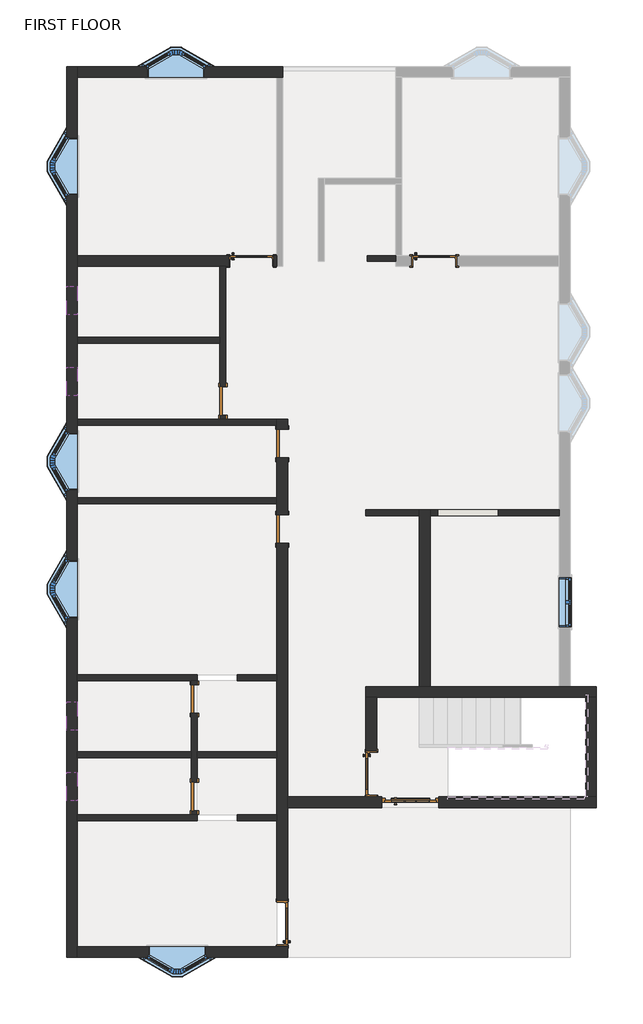
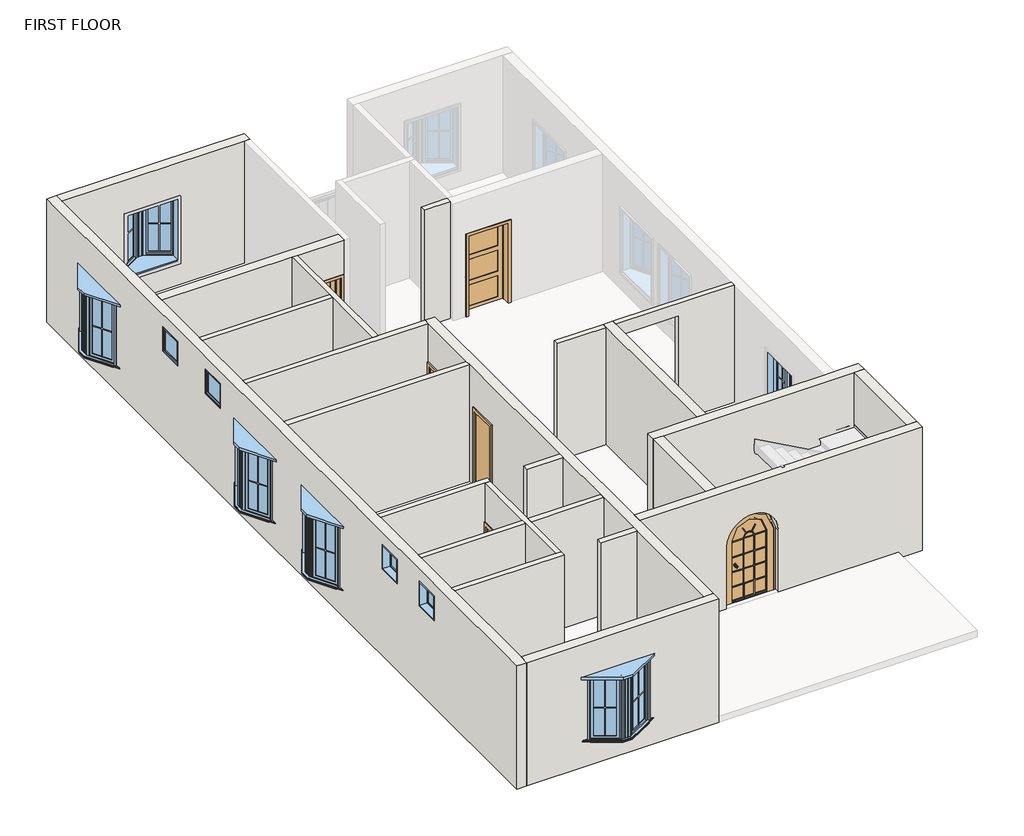
# One storey, part 1 of 2: 23 walls, 10 doors, 10 windows.
"""IFC4 building model written with IfcOpenShell, lengths in millimetres."""

from ifc_helpers import new_model, si_unit, frame, origin, place, context, project, spatial, polyline, circle_curve, outline, extrude, faceted_brep, transform, mapped, element, save
from ifc_brep_helpers import plane_surface, revolved_surface, advanced_brep
from components import door_interior_single_3_panel_vert_wood_interior_door_3_x_7_9905b5e2, door_interior_single_3_panel_vert_wood_interior_door_3_x_7_d98c575a, door_arched_single_french_glass_wood_exterior_1219_x_2134mm_7a906126, single_flush_bathroom_flush_door_2_x_7_025d1c86, single_flush_bathroom_flush_door_2_x_7_11f1894d, single_flush_bathroom_flush_door_2_x_7_88cc3d71, window_80340324, window_bay_casement_30_degree_angle_30_angle_window_doors_2_b97d1700, window_c95ebb39

model = new_model("IFC4")

# Units and contexts
model_context = context("Model", 3, world=origin())
ifc_project = project(units=[si_unit("LENGTHUNIT", "METRE", prefix="MILLI")], contexts=[model_context])

# Site, building, storey
site = spatial("IfcSite", under=ifc_project)
building = spatial("IfcBuilding", under=site)
storey = spatial("IfcBuildingStorey", under=building, Name="FIRST FLOOR", Elevation=3352.8)

# Doors
placement = place(None, origin())
door_interior_single_3_panel_vert_wood_interior_door_3_x_7_shape = door_interior_single_3_panel_vert_wood_interior_door_3_x_7_9905b5e2(model_context)
element("IfcDoor", 1, ObjectType="Door-Interior-Single-3_Panel_Vert-Wood : INTERIOR DOOR 3' X 7'", at=placement, inside=storey, context=model_context, shape_type="MappedRepresentation", body=[
    mapped(door_interior_single_3_panel_vert_wood_interior_door_3_x_7_shape, transform((-12438.2436606, 7459.3725873, 3352.8), x_axis=(1.0, 0.0, 0.0), y_axis=(0.0, 1.0, 0.0), z_axis=(0.0, 0.0, 1.0))),
])
element("IfcDoor", 2, ObjectType="Door-Interior-Single-3_Panel_Vert-Wood : INTERIOR DOOR 3' X 7'", at=placement, inside=storey, context=model_context, shape_type="MappedRepresentation", body=[
    mapped(door_interior_single_3_panel_vert_wood_interior_door_3_x_7_shape, transform((-16349.8436606, 7459.3725873, 3352.8), x_axis=(1.0, 0.0, 0.0), y_axis=(0.0, 1.0, 0.0), z_axis=(0.0, 0.0, 1.0))),
])
door_interior_single_3_panel_vert_wood_interior_door_3_x_7_2_shape = door_interior_single_3_panel_vert_wood_interior_door_3_x_7_d98c575a(model_context)
element("IfcDoor", 3, ObjectType="Door-Interior-Single-3_Panel_Vert-Wood : INTERIOR DOOR 3' X 7'", at=placement, inside=storey, context=model_context, shape_type="MappedRepresentation", body=[
    mapped(door_interior_single_3_panel_vert_wood_interior_door_3_x_7_2_shape, transform((-15686.2686606, -6717.0024127, 3352.8), x_axis=(0.0, 1.0, 0.0), y_axis=(-1.0, 0.0, 0.0), z_axis=(0.0, 0.0, 1.0))),
])
element("IfcDoor", 4, ObjectType="Door-Interior-Single-3_Panel_Vert-Wood : INTERIOR DOOR 3' X 7'", at=placement, inside=storey, context=model_context, shape_type="MappedRepresentation", body=[
    mapped(door_interior_single_3_panel_vert_wood_interior_door_3_x_7_2_shape, transform((-13787.6186606, -3516.6024127, 3352.8), x_axis=(0.0, -1.0, 0.0), y_axis=(1.0, 0.0, 0.0), z_axis=(0.0, 0.0, 1.0))),
])
door_arched_single_french_glass_wood_exterior_1219_x_2134mm_shape = door_arched_single_french_glass_wood_exterior_1219_x_2134mm_7a906126(model_context)
element("IfcDoor", 5, ObjectType="Door_Arched_Single_French_Glass_Wood_Exterior : 1219 x 2134mm", at=placement, inside=storey, context=model_context, shape_type="MappedRepresentation", body=[
    mapped(door_arched_single_french_glass_wood_exterior_1219_x_2134mm_shape, transform((-12946.2436606, -4126.2024127, 3352.8), x_axis=(1.0, 0.0, 0.0), y_axis=(0.0, 1.0, 0.0), z_axis=(0.0, 0.0, 1.0))),
])
single_flush_bathroom_flush_door_2_x_7_shape = single_flush_bathroom_flush_door_2_x_7_025d1c86(model_context)
element("IfcDoor", 6, ObjectType="Single-Flush : BATHROOM FLUSH DOOR 2' X 7'", at=placement, inside=storey, context=model_context, shape_type="MappedRepresentation", body=[
    mapped(single_flush_bathroom_flush_door_2_x_7_shape, transform((-16959.4436606, 4458.9975873, 3352.8), x_axis=(0.0, 1.0, 0.0), y_axis=(-1.0, 0.0, 0.0), z_axis=(0.0, 0.0, 1.0))),
])
element("IfcDoor", 7, ObjectType="Single-Flush : BATHROOM FLUSH DOOR 2' X 7'", at=placement, inside=storey, context=model_context, shape_type="MappedRepresentation", body=[
    mapped(single_flush_bathroom_flush_door_2_x_7_shape, transform((-17569.0436606, -1916.4024127, 3352.8), x_axis=(0.0, 1.0, 0.0), y_axis=(-1.0, 0.0, 0.0), z_axis=(0.0, 0.0, 1.0))),
])
element("IfcDoor", 8, ObjectType="Single-Flush : BATHROOM FLUSH DOOR 2' X 7'", at=placement, inside=storey, context=model_context, shape_type="MappedRepresentation", body=[
    mapped(single_flush_bathroom_flush_door_2_x_7_shape, transform((-17569.0436606, -3999.2024127, 3352.8), x_axis=(0.0, 1.0, 0.0), y_axis=(-1.0, 0.0, 0.0), z_axis=(0.0, 0.0, 1.0))),
])
single_flush_bathroom_flush_door_2_x_7_2_shape = single_flush_bathroom_flush_door_2_x_7_11f1894d(model_context)
element("IfcDoor", 9, ObjectType="Single-Flush : BATHROOM FLUSH DOOR 2' X 7'", at=placement, inside=storey, context=model_context, shape_type="MappedRepresentation", body=[
    mapped(single_flush_bathroom_flush_door_2_x_7_2_shape, transform((-15689.4436606, 1715.7975873, 3352.8), x_axis=(0.0, -1.0, 0.0), y_axis=(1.0, 0.0, 0.0), z_axis=(0.0, 0.0, 1.0))),
])
single_flush_bathroom_flush_door_2_x_7_3_shape = single_flush_bathroom_flush_door_2_x_7_88cc3d71(model_context)
element("IfcDoor", 10, ObjectType="Single-Flush : BATHROOM FLUSH DOOR 2' X 7'", at=placement, inside=storey, context=model_context, shape_type="MappedRepresentation", body=[
    mapped(single_flush_bathroom_flush_door_2_x_7_3_shape, transform((-15689.4436606, 3544.5975873, 3352.8), x_axis=(0.0, 1.0, 0.0), y_axis=(-1.0, 0.0, 0.0), z_axis=(0.0, 0.0, 1.0))),
])

# Walls
element("IfcWall", 11, at=placement, inside=storey, context=model_context, shape_type="Brep", body=[
    faceted_brep([(-20299.5436606, 11609.0975873, 3352.8), (-20299.5436606, -7440.9024127, 3352.8), (-20299.5436606, -7440.9024127, 6400.8), (-20299.5436606, 11609.0975873, 6400.8), (-20299.5436606, 1077.6225873, 5537.2), (-20299.5436606, -211.4274127, 5537.2), (-20299.5436606, -211.4274127, 3962.4), (-20299.5436606, 1077.6225873, 3962.4), (-20299.5436606, 3808.1225873, 5537.2), (-20299.5436606, 2519.0725873, 5537.2), (-20299.5436606, 2519.0725873, 3962.4), (-20299.5436606, 3808.1225873, 3962.4), (-20299.5436606, 10120.0225873, 5537.2), (-20299.5436606, 8830.9725873, 5537.2), (-20299.5436606, 8830.9725873, 3962.4), (-20299.5436606, 10120.0225873, 3962.4), (-20299.5436606, -2589.5024127, 6096.0), (-20299.5436606, -2589.5024127, 5486.4), (-20299.5436606, -1979.9024127, 5486.4), (-20299.5436606, -1979.9024127, 6096.0), (-20299.5436606, -4088.1024127, 6096.0), (-20299.5436606, -4088.1024127, 5486.4), (-20299.5436606, -3478.5024127, 5486.4), (-20299.5436606, -3478.5024127, 6096.0), (-20299.5436606, 5182.8975873, 6096.0), (-20299.5436606, 4573.2975873, 6096.0), (-20299.5436606, 4573.2975873, 5486.4), (-20299.5436606, 5182.8975873, 5486.4), (-20299.5436606, 6910.0975873, 6096.0), (-20299.5436606, 6300.4975873, 6096.0), (-20299.5436606, 6300.4975873, 5486.4), (-20299.5436606, 6910.0975873, 5486.4), (-20070.9436606, 11609.0975873, 3352.8), (-20070.9436606, 11609.0975873, 6400.8), (-20070.9436606, 11380.4975873, 6400.8), (-20070.9436606, 7570.4975873, 6400.8), (-20070.9436606, 7341.8975873, 6400.8), (-20070.9436606, 5817.8975873, 6400.8), (-20070.9436606, 5690.8975873, 6400.8), (-20070.9436606, 4065.2975873, 6400.8), (-20070.9436606, 3938.2975873, 6400.8), (-20070.9436606, 2388.8975873, 6400.8), (-20070.9436606, 2261.8975873, 6400.8), (-20070.9436606, -1395.7024127, 6400.8), (-20070.9436606, -1522.7024127, 6400.8), (-20070.9436606, -3046.7024127, 6400.8), (-20070.9436606, -3173.7024127, 6400.8), (-20070.9436606, -4392.9024127, 6400.8), (-20070.9436606, -4519.9024127, 6400.8), (-20070.9436606, -7212.3024127, 6400.8), (-20070.9436606, -7440.9024127, 6400.8), (-20070.9436606, -7440.9024127, 3352.8), (-20070.9436606, -7212.3024127, 3352.8), (-20070.9436606, -4519.9024127, 3352.8), (-20070.9436606, -4392.9024127, 3352.8), (-20070.9436606, -3173.7024127, 3352.8), (-20070.9436606, -3046.7024127, 3352.8), (-20070.9436606, -1522.7024127, 3352.8), (-20070.9436606, -1395.7024127, 3352.8), (-20070.9436606, 2261.8975873, 3352.8), (-20070.9436606, 2388.8975873, 3352.8), (-20070.9436606, 3938.2975873, 3352.8), (-20070.9436606, 4065.2975873, 3352.8), (-20070.9436606, 5690.8975873, 3352.8), (-20070.9436606, 5817.8975873, 3352.8), (-20070.9436606, 7341.8975873, 3352.8), (-20070.9436606, 7570.4975873, 3352.8), (-20070.9436606, 11380.4975873, 3352.8), (-20070.9436606, -176.5024127, 5537.2), (-20070.9436606, 1042.6975873, 5537.2), (-20070.9436606, 1042.6975873, 3962.4), (-20070.9436606, -176.5024127, 3962.4), (-20070.9436606, 2553.9975873, 5537.2), (-20070.9436606, 3773.1975873, 5537.2), (-20070.9436606, 3773.1975873, 3962.4), (-20070.9436606, 2553.9975873, 3962.4), (-20070.9436606, 8865.8975873, 5537.2), (-20070.9436606, 10085.0975873, 5537.2), (-20070.9436606, 10085.0975873, 3962.4), (-20070.9436606, 8865.8975873, 3962.4), (-20070.9436606, -2589.5024127, 6096.0), (-20070.9436606, -1979.9024127, 6096.0), (-20070.9436606, -1979.9024127, 5486.4), (-20070.9436606, -2589.5024127, 5486.4), (-20070.9436606, -4088.1024127, 6096.0), (-20070.9436606, -3478.5024127, 6096.0), (-20070.9436606, -3478.5024127, 5486.4), (-20070.9436606, -4088.1024127, 5486.4), (-20070.9436606, 5182.8975873, 6096.0), (-20070.9436606, 5182.8975873, 5486.4), (-20070.9436606, 4573.2975873, 5486.4), (-20070.9436606, 4573.2975873, 6096.0), (-20070.9436606, 6910.0975873, 6096.0), (-20070.9436606, 6910.0975873, 5486.4), (-20070.9436606, 6300.4975873, 5486.4), (-20070.9436606, 6300.4975873, 6096.0), (-20239.0517862, -176.5024127, 5537.2), (-20239.0517862, 1042.6975873, 5537.2), (-20239.0517862, -176.5024127, 3962.4), (-20239.0517862, 1042.6975873, 3962.4), (-20239.0517862, 2553.9975873, 5537.2), (-20239.0517862, 3773.1975873, 5537.2), (-20239.0517862, 2553.9975873, 3962.4), (-20239.0517862, 3773.1975873, 3962.4), (-20239.0517862, 8865.8975873, 5537.2), (-20239.0517862, 10085.0975873, 5537.2), (-20239.0517862, 8865.8975873, 3962.4), (-20239.0517862, 10085.0975873, 3962.4)], [[[0, 1, 2, 3], [4, 5, 6, 7], [8, 9, 10, 11], [12, 13, 14, 15], [16, 17, 18, 19], [20, 21, 22, 23], [24, 25, 26, 27], [28, 29, 30, 31]], [[32, 33, 34, 35, 36, 37, 38, 39, 40, 41, 42, 43, 44, 45, 46, 47, 48, 49, 50, 51, 52, 53, 54, 55, 56, 57, 58, 59, 60, 61, 62, 63, 64, 65, 66, 67], [68, 69, 70, 71], [72, 73, 74, 75], [76, 77, 78, 79], [80, 81, 82, 83], [84, 85, 86, 87], [88, 89, 90, 91], [92, 93, 94, 95]], [[1, 0, 32, 67, 66, 65, 64, 63, 62, 61, 60, 59, 58, 57, 56, 55, 54, 53, 52, 51]], [[3, 2, 50, 49, 48, 47, 46, 45, 44, 43, 42, 41, 40, 39, 38, 37, 36, 35, 34, 33]], [[2, 1, 51, 50]], [[0, 3, 33, 32]], [[96, 5, 4, 97, 69, 68]], [[98, 71, 70, 99, 7, 6]], [[96, 68, 71, 98]], [[69, 97, 99, 70]], [[97, 4, 7, 99]], [[5, 96, 98, 6]], [[100, 9, 8, 101, 73, 72]], [[102, 75, 74, 103, 11, 10]], [[100, 72, 75, 102]], [[73, 101, 103, 74]], [[101, 8, 11, 103]], [[9, 100, 102, 10]], [[104, 13, 12, 105, 77, 76]], [[106, 79, 78, 107, 15, 14]], [[104, 76, 79, 106]], [[77, 105, 107, 78]], [[105, 12, 15, 107]], [[13, 104, 106, 14]], [[17, 16, 80, 83]], [[18, 17, 83, 82]], [[19, 18, 82, 81]], [[16, 19, 81, 80]], [[21, 20, 84, 87]], [[22, 21, 87, 86]], [[23, 22, 86, 85]], [[20, 23, 85, 84]], [[89, 88, 24, 27]], [[90, 89, 27, 26]], [[91, 90, 26, 25]], [[88, 91, 25, 24]], [[93, 92, 28, 31]], [[94, 93, 31, 30]], [[95, 94, 30, 29]], [[92, 95, 29, 28]]]),
])
element("IfcWall", 12, at=placement, inside=storey, context=model_context, shape_type="Brep", body=[
    faceted_brep([(-20070.9436606, -7440.9024127, 3352.8), (-15575.1436606, -7440.9024127, 3352.8), (-15575.1436606, -7440.9024127, 6400.8), (-20070.9436606, -7440.9024127, 6400.8), (-18581.8686606, -7440.9024127, 5537.2), (-17292.8186606, -7440.9024127, 5537.2), (-17292.8186606, -7440.9024127, 3962.4), (-18581.8686606, -7440.9024127, 3962.4), (-20070.9436606, -7212.3024127, 3352.8), (-20070.9436606, -7212.3024127, 6400.8), (-15803.7436606, -7212.3024127, 6400.8), (-15575.1436606, -7212.3024127, 6400.8), (-15575.1436606, -7212.3024127, 3352.8), (-15803.7436606, -7212.3024127, 3352.8), (-17327.7436606, -7212.3024127, 5537.2), (-18546.9436606, -7212.3024127, 5537.2), (-18546.9436606, -7212.3024127, 3962.4), (-17327.7436606, -7212.3024127, 3962.4), (-17327.7436606, -7380.4105382, 5537.2), (-18546.9436606, -7380.4105382, 5537.2), (-17327.7436606, -7380.4105382, 3962.4), (-18546.9436606, -7380.4105382, 3962.4)], [[[0, 1, 2, 3], [4, 5, 6, 7]], [[8, 9, 10, 11, 12, 13], [14, 15, 16, 17]], [[1, 0, 8, 13, 12]], [[3, 2, 11, 10, 9]], [[0, 3, 9, 8]], [[2, 1, 12, 11]], [[18, 5, 4, 19, 15, 14]], [[20, 17, 16, 21, 7, 6]], [[18, 14, 17, 20]], [[15, 19, 21, 16]], [[19, 4, 7, 21]], [[5, 18, 20, 6]]]),
])
element("IfcWall", 13, at=placement, inside=storey, context=model_context, shape_type="Brep", body=[
    faceted_brep([(-15575.1436606, 4065.2975873, 6400.8), (-15575.1436606, -4011.9024127, 6400.8), (-15575.1436606, -4240.5024127, 6400.8), (-15575.1436606, -7212.3024127, 6400.8), (-15575.1436606, -7212.3024127, 3352.8), (-15575.1436606, -7199.6024127, 3352.8), (-15575.1436606, -7199.6024127, 5511.8), (-15575.1436606, -6234.4024127, 5511.8), (-15575.1436606, -6234.4024127, 3352.8), (-15575.1436606, -4240.5024127, 3352.8), (-15575.1436606, -4011.9024127, 3352.8), (-15575.1436606, 1410.9975873, 3352.8), (-15575.1436606, 1410.9975873, 5384.8), (-15575.1436606, 2020.5975873, 5384.8), (-15575.1436606, 2020.5975873, 3352.8), (-15575.1436606, 3239.7975873, 3352.8), (-15575.1436606, 3239.7975873, 5384.8), (-15575.1436606, 3849.3975873, 5384.8), (-15575.1436606, 3849.3975873, 3352.8), (-15575.1436606, 4065.2975873, 3352.8), (-15803.7436606, -7212.3024127, 6400.8), (-15803.7436606, -4519.9024127, 6400.8), (-15803.7436606, -4392.9024127, 6400.8), (-15803.7436606, -3173.7024127, 6400.8), (-15803.7436606, -3046.7024127, 6400.8), (-15803.7436606, -1522.7024127, 6400.8), (-15803.7436606, -1395.7024127, 6400.8), (-15803.7436606, 2261.8975873, 6400.8), (-15803.7436606, 2388.8975873, 6400.8), (-15803.7436606, 3938.2975873, 6400.8), (-15803.7436606, 4065.2975873, 6400.8), (-15803.7436606, 4065.2975873, 3352.8), (-15803.7436606, 3938.2975873, 3352.8), (-15803.7436606, 3849.3975873, 3352.8), (-15803.7436606, 3849.3975873, 5384.8), (-15803.7436606, 3239.7975873, 5384.8), (-15803.7436606, 3239.7975873, 3352.8), (-15803.7436606, 2388.8975873, 3352.8), (-15803.7436606, 2261.8975873, 3352.8), (-15803.7436606, 2020.5975873, 3352.8), (-15803.7436606, 2020.5975873, 5384.8), (-15803.7436606, 1410.9975873, 5384.8), (-15803.7436606, 1410.9975873, 3352.8), (-15803.7436606, -1395.7024127, 3352.8), (-15803.7436606, -1522.7024127, 3352.8), (-15803.7436606, -3046.7024127, 3352.8), (-15803.7436606, -3173.7024127, 3352.8), (-15803.7436606, -4392.9024127, 3352.8), (-15803.7436606, -4519.9024127, 3352.8), (-15803.7436606, -6234.4024127, 3352.8), (-15803.7436606, -6234.4024127, 5511.8), (-15803.7436606, -7199.6024127, 5511.8), (-15803.7436606, -7199.6024127, 3352.8), (-15803.7436606, -7212.3024127, 3352.8)], [[[0, 1, 2, 3, 4, 5, 6, 7, 8, 9, 10, 11, 12, 13, 14, 15, 16, 17, 18, 19]], [[20, 21, 22, 23, 24, 25, 26, 27, 28, 29, 30, 31, 32, 33, 34, 35, 36, 37, 38, 39, 40, 41, 42, 43, 44, 45, 46, 47, 48, 49, 50, 51, 52, 53]], [[4, 53, 52, 5]], [[31, 19, 18, 33, 32]], [[42, 11, 10, 9, 8, 49, 48, 47, 46, 45, 44, 43]], [[14, 39, 38, 37, 36, 15]], [[3, 2, 1, 0, 30, 29, 28, 27, 26, 25, 24, 23, 22, 21, 20]], [[4, 3, 20, 53]], [[0, 19, 31, 30]], [[41, 12, 11, 42]], [[40, 13, 12, 41]], [[13, 40, 39, 14]], [[34, 33, 18, 17]], [[35, 34, 17, 16]], [[36, 35, 16, 15]], [[7, 50, 49, 8]], [[50, 7, 6, 51]], [[51, 6, 5, 52]]]),
])
element("IfcWall", 14, at=placement, inside=storey, context=model_context, shape_type="Brep", body=[
    faceted_brep([(-15803.7436606, 7341.8975873, 6400.8), (-16895.9436606, 7341.8975873, 6400.8), (-17022.9436606, 7341.8975873, 6400.8), (-20070.9436606, 7341.8975873, 6400.8), (-20070.9436606, 7341.8975873, 3352.8), (-17022.9436606, 7341.8975873, 3352.8), (-16895.9436606, 7341.8975873, 3352.8), (-16832.4436606, 7341.8975873, 3352.8), (-16832.4436606, 7341.8975873, 5511.8), (-15867.2436606, 7341.8975873, 5511.8), (-15867.2436606, 7341.8975873, 3352.8), (-15803.7436606, 7341.8975873, 3352.8), (-20070.9436606, 7570.4975873, 6400.8), (-15803.7436606, 7570.4975873, 6400.8), (-15803.7436606, 7570.4975873, 3352.8), (-15867.2436606, 7570.4975873, 3352.8), (-15867.2436606, 7570.4975873, 5511.8), (-16832.4436606, 7570.4975873, 5511.8), (-16832.4436606, 7570.4975873, 3352.8), (-20070.9436606, 7570.4975873, 3352.8)], [[[0, 1, 2, 3, 4, 5, 6, 7, 8, 9, 10, 11]], [[12, 13, 14, 15, 16, 17, 18, 19]], [[4, 19, 18, 7, 6, 5]], [[14, 11, 10, 15]], [[3, 2, 1, 0, 13, 12]], [[4, 3, 12, 19]], [[0, 11, 14, 13]], [[9, 16, 15, 10]], [[16, 9, 8, 17]], [[17, 8, 7, 18]]]),
])
element("IfcWall", 15, at=placement, inside=storey, context=model_context, shape_type="Brep", body=[
    faceted_brep([(-20070.9436606, 11380.4975873, 3352.8), (-15803.7436606, 11380.4975873, 3352.8), (-15676.7436606, 11380.4975873, 3352.8), (-15676.7436606, 11380.4975873, 6400.8), (-15803.7436606, 11380.4975873, 6400.8), (-20070.9436606, 11380.4975873, 6400.8), (-18572.3436606, 11380.4975873, 5537.2), (-17353.1436606, 11380.4975873, 5537.2), (-17353.1436606, 11380.4975873, 3962.4), (-18572.3436606, 11380.4975873, 3962.4), (-20070.9436606, 11609.0975873, 3352.8), (-20070.9436606, 11609.0975873, 6400.8), (-15676.7436606, 11609.0975873, 6400.8), (-15676.7436606, 11609.0975873, 3352.8), (-17318.2186606, 11609.0975873, 5537.2), (-18607.2686606, 11609.0975873, 5537.2), (-18607.2686606, 11609.0975873, 3962.4), (-17318.2186606, 11609.0975873, 3962.4), (-18572.3436606, 11548.6057128, 5537.2), (-17353.1436606, 11548.6057128, 5537.2), (-18572.3436606, 11548.6057128, 3962.4), (-17353.1436606, 11548.6057128, 3962.4)], [[[0, 1, 2, 3, 4, 5], [6, 7, 8, 9]], [[10, 11, 12, 13], [14, 15, 16, 17]], [[2, 1, 0, 10, 13]], [[5, 4, 3, 12, 11]], [[0, 5, 11, 10]], [[3, 2, 13, 12]], [[18, 15, 14, 19, 7, 6]], [[20, 9, 8, 21, 17, 16]], [[18, 6, 9, 20]], [[7, 19, 21, 8]], [[19, 14, 17, 21]], [[15, 18, 20, 16]]]),
])
element("IfcWall", 16, at=placement, inside=storey, context=model_context, shape_type="Brep", body=[
    faceted_brep([(-8971.1436606, -1649.7024127, 3352.8), (-9529.9436606, -1649.7024127, 3352.8), (-9758.5436606, -1649.7024127, 3352.8), (-12527.1436606, -1649.7024127, 3352.8), (-12755.7436606, -1649.7024127, 3352.8), (-13898.7436606, -1649.7024127, 3352.8), (-13898.7436606, -1649.7024127, 6400.8), (-12755.7436606, -1649.7024127, 6400.8), (-12527.1436606, -1649.7024127, 6400.8), (-9758.5436606, -1649.7024127, 6400.8), (-9529.9436606, -1649.7024127, 6400.8), (-8971.1436606, -1649.7024127, 6400.8), (-8971.1436606, -1878.3024127, 3352.8), (-8971.1436606, -1878.3024127, 6400.8), (-9199.7436606, -1878.3024127, 6400.8), (-13670.1436606, -1878.3024127, 6400.8), (-13898.7436606, -1878.3024127, 6400.8), (-13898.7436606, -1878.3024127, 3352.8), (-13670.1436606, -1878.3024127, 3352.8), (-9199.7436606, -1878.3024127, 3352.8)], [[[0, 1, 2, 3, 4, 5, 6, 7, 8, 9, 10, 11]], [[12, 13, 14, 15, 16, 17, 18, 19]], [[5, 4, 3, 2, 1, 0, 12, 19, 18, 17]], [[11, 10, 9, 8, 7, 6, 16, 15, 14, 13]], [[6, 5, 17, 16]], [[0, 11, 13, 12]]]),
])
element("IfcWall", 17, at=placement, inside=storey, context=model_context, shape_type="SweptSolid", body=[
    extrude(outline(polyline([(-4011.9024127, 6400.8), (-1878.3024127, 6400.8), (-1878.3024127, 3352.8), (-3034.0024127, 3352.8), (-3034.0024127, 5511.8), (-3999.2024127, 5511.8), (-3999.2024127, 3352.8), (-4011.9024127, 3352.8), (-4011.9024127, 6400.8)])), frame((-13898.7436606, 0.0, 0.0), z_axis=(1.0, 0.0, 0.0), x_axis=(0.0, 1.0, 0.0)), (0.0, 0.0, 1.0), 228.6),
])
element("IfcWall", 18, at=placement, inside=storey, context=model_context, shape_type="Brep", body=[
    faceted_brep([(-12527.1436606, -1649.7024127, 3352.8), (-12527.1436606, 2007.8975873, 3352.8), (-12527.1436606, 2134.8975873, 3352.8), (-12527.1436606, 2134.8975873, 6400.8), (-12527.1436606, 2007.8975873, 6400.8), (-12527.1436606, -1649.7024127, 6400.8), (-12755.7436606, -1649.7024127, 3352.8), (-12755.7436606, -1649.7024127, 6400.8), (-12755.7436606, 2007.8975873, 6400.8), (-12755.7436606, 2134.8975873, 6400.8), (-12755.7436606, 2134.8975873, 3352.8), (-12755.7436606, 2007.8975873, 3352.8)], [[[0, 1, 2, 3, 4, 5]], [[6, 7, 8, 9, 10, 11]], [[2, 1, 0, 6, 11, 10]], [[5, 4, 3, 9, 8, 7]], [[0, 5, 7, 6]], [[3, 2, 10, 9]]]),
])
element("IfcWall", 19, at=placement, inside=storey, context=model_context, shape_type="AdvancedBrep", body=[
    advanced_brep(
    [(-12336.6436606, -4240.5024127, 5031.4), (-12336.6436606, -4240.5024127, 3352.8), (-8971.1436606, -4240.5024127, 3352.8), (-8971.1436606, -4240.5024127, 6400.8), (-15575.1436606, -4240.5024127, 6400.8), (-15575.1436606, -4240.5024127, 3352.8), (-13555.8436606, -4240.5024127, 3352.8), (-13555.8436606, -4240.5024127, 5031.4), (-8971.1436606, -4011.9024127, 3352.8), (-9199.7436606, -4011.9024127, 3352.8), (-12336.6436606, -4011.9024127, 3352.8), (-12336.6436606, -4011.9024127, 5031.4), (-13555.8436606, -4011.9024127, 5031.4), (-13555.8436606, -4011.9024127, 3352.8), (-13670.1436606, -4011.9024127, 3352.8), (-13898.7436606, -4011.9024127, 3352.8), (-15575.1436606, -4011.9024127, 3352.8), (-15575.1436606, -4011.9024127, 6400.8), (-13898.7436606, -4011.9024127, 6400.8), (-13670.1436606, -4011.9024127, 6400.8), (-9199.7436606, -4011.9024127, 6400.8), (-8971.1436606, -4011.9024127, 6400.8)],
    [
        (0, 1),
        (1, 2),
        (2, 3),
        (3, 4),
        (4, 5),
        (5, 6),
        (6, 7),
        (7, 0, circle_curve(frame((-12946.2436606, -4240.5024127, 5031.4), z_axis=(0.0, 1.0, 0.0), x_axis=(1.0, 0.0, 0.0)), 609.6)),
        (8, 9),
        (9, 10),
        (10, 11),
        (11, 12, circle_curve(frame((-12946.2436606, -4011.9024127, 5031.4), z_axis=(0.0, -1.0, 0.0), x_axis=(1.0, 0.0, 0.0)), 609.6)),
        (12, 13),
        (13, 14),
        (14, 15),
        (15, 16),
        (16, 17),
        (17, 18),
        (18, 19),
        (19, 20),
        (20, 21),
        (21, 8),
        (5, 16),
        (13, 6),
        (1, 10),
        (8, 2),
        (3, 21),
        (17, 4),
        (11, 0),
        (7, 12),
    ],
    [
        plane_surface(frame((-15565.8912748, -4240.5024127, 3352.8), z_axis=(0.0, -1.0, 0.0), x_axis=(1.0, 0.0, 0.0))),
        plane_surface(frame((-15565.8912748, -4011.9024127, 3352.8), z_axis=(0.0, 1.0, 0.0), x_axis=(-1.0, 0.0, 0.0))),
        plane_surface(frame((-15689.4436606, -4240.5024127, 3352.8), z_axis=(0.0, 0.0, -1.0), x_axis=(0.0, 1.0, 0.0))),
        plane_surface(frame((-9085.4436606, -4240.5024127, 6400.8), z_axis=(0.0, 0.0, 1.0), x_axis=(0.0, 1.0, 0.0))),
        plane_surface(frame((-15575.1436606, -7212.3024127, 3352.8), z_axis=(-1.0, 0.0, 0.0), x_axis=(0.0, 1.0, 0.0))),
        plane_surface(frame((-8971.1436606, -4011.9024127, 3352.8), z_axis=(1.0, 0.0, 0.0), x_axis=(0.0, 1.0, 0.0))),
        revolved_surface(polyline([(-12336.643660599999, -4240.5024127, 5031.4), (-12336.643660599999, -4011.9024127, 5031.4)]), (-12946.2436606, -4240.5024127, 5031.4), (0.0, -1.0, 0.0)),
        plane_surface(frame((-13555.8436606, -4011.9024127, 5031.4), z_axis=(1.0, 0.0, 0.0), x_axis=(0.0, -1.0, 0.0))),
        plane_surface(frame((-12336.6436606, -4011.9024127, 3352.8), z_axis=(-1.0, 0.0, 0.0), x_axis=(0.0, -1.0, 0.0))),
    ],
    [
        (0, [[1, 2, 3, 4, 5, 6, 7, 8]]),
        (1, [[9, 10, 11, 12, 13, 14, 15, 16, 17, 18, 19, 20, 21, 22]]),
        (2, [[-6, 23, -16, -15, -14, 24]]),
        (2, [[-2, 25, -10, -9, 26]]),
        (3, [[-4, 27, -21, -20, -19, -18, 28]]),
        (4, [[-5, -28, -17, -23]]),
        (5, [[-3, -26, -22, -27]]),
        (6, [[-12, 29, -8, 30]]),
        (7, [[-13, -30, -7, -24]]),
        (8, [[-11, -25, -1, -29]]),
    ],
),
])
element("IfcWall", 20, at=placement, inside=storey, context=model_context, shape_type="SweptSolid", body=[
    extrude(outline(polyline([(-8971.1436606, -1878.3024127), (-8971.1436606, -4011.9024127), (-9199.7436606, -4011.9024127), (-9199.7436606, -1878.3024127), (-8971.1436606, -1878.3024127)])), frame((0.0, 0.0, 3352.8), z_axis=(0.0, 0.0, 1.0), x_axis=(1.0, 0.0, 0.0)), (0.0, 0.0, 1.0), 3048.0),
])
element("IfcWall", 21, ObjectType="INNER WALL 5\"", at=placement, inside=storey, context=model_context, shape_type="SweptSolid", body=[
    extrude(outline(polyline([(-13263.7436606, 7443.4975873), (-13873.3436606, 7443.4975873), (-13873.3436606, 7570.4975873), (-13263.7436606, 7570.4975873), (-13263.7436606, 7443.4975873)])), frame((0.0, 0.0, 3352.8), z_axis=(0.0, 0.0, 1.0), x_axis=(1.0, 0.0, 0.0)), (0.0, 0.0, 1.0), 3048.0),
])
element("IfcWall", 22, ObjectType="INNER WALL 5\"", at=placement, inside=storey, context=model_context, shape_type="Brep", body=[
    faceted_brep([(-17022.9436606, 7341.8975873, 3352.8), (-17022.9436606, 5817.8975873, 3352.8), (-17022.9436606, 5690.8975873, 3352.8), (-17022.9436606, 4763.7975873, 3352.8), (-17022.9436606, 4763.7975873, 5384.8), (-17022.9436606, 4154.1975873, 5384.8), (-17022.9436606, 4154.1975873, 3352.8), (-17022.9436606, 4065.2975873, 3352.8), (-17022.9436606, 4065.2975873, 6400.8), (-17022.9436606, 5690.8975873, 6400.8), (-17022.9436606, 5817.8975873, 6400.8), (-17022.9436606, 7341.8975873, 6400.8), (-16895.9436606, 4763.7975873, 5384.8), (-16895.9436606, 4763.7975873, 3352.8), (-16895.9436606, 7341.8975873, 3352.8), (-16895.9436606, 7341.8975873, 6400.8), (-16895.9436606, 4065.2975873, 6400.8), (-16895.9436606, 4065.2975873, 3352.8), (-16895.9436606, 4154.1975873, 3352.8), (-16895.9436606, 4154.1975873, 5384.8)], [[[0, 1, 2, 3, 4, 5, 6, 7, 8, 9, 10, 11]], [[12, 13, 14, 15, 16, 17, 18, 19]], [[18, 17, 7, 6]], [[14, 13, 3, 2, 1, 0]], [[11, 10, 9, 8, 16, 15]], [[0, 11, 15, 14]], [[8, 7, 17, 16]], [[4, 3, 13, 12]], [[5, 4, 12, 19]], [[6, 5, 19, 18]]]),
])
element("IfcWall", 23, ObjectType="INNER WALL 5\"", at=placement, inside=storey, context=model_context, shape_type="SweptSolid", body=[
    extrude(outline(polyline([(-17022.9436606, 5690.8975873), (-20070.9436606, 5690.8975873), (-20070.9436606, 5817.8975873), (-17022.9436606, 5817.8975873), (-17022.9436606, 5690.8975873)])), frame((0.0, 0.0, 3352.8), z_axis=(0.0, 0.0, 1.0), x_axis=(1.0, 0.0, 0.0)), (0.0, 0.0, 1.0), 3048.0),
])
element("IfcWall", 24, ObjectType="INNER WALL 5\"", at=placement, inside=storey, context=model_context, shape_type="Brep", body=[
    faceted_brep([(-15803.7436606, 4065.2975873, 3352.8), (-16895.9436606, 4065.2975873, 3352.8), (-17022.9436606, 4065.2975873, 3352.8), (-20070.9436606, 4065.2975873, 3352.8), (-20070.9436606, 4065.2975873, 6400.8), (-17022.9436606, 4065.2975873, 6400.8), (-16895.9436606, 4065.2975873, 6400.8), (-15803.7436606, 4065.2975873, 6400.8), (-15803.7436606, 3938.2975873, 3352.8), (-15803.7436606, 3938.2975873, 6400.8), (-20070.9436606, 3938.2975873, 6400.8), (-20070.9436606, 3938.2975873, 3352.8)], [[[0, 1, 2, 3, 4, 5, 6, 7]], [[8, 9, 10, 11]], [[3, 2, 1, 0, 8, 11]], [[7, 6, 5, 4, 10, 9]], [[0, 7, 9, 8]], [[4, 3, 11, 10]]]),
])
element("IfcWall", 25, ObjectType="INNER WALL 5\"", at=placement, inside=storey, context=model_context, shape_type="SweptSolid", body=[
    extrude(outline(polyline([(-15803.7436606, 2261.8975873), (-20070.9436606, 2261.8975873), (-20070.9436606, 2388.8975873), (-15803.7436606, 2388.8975873), (-15803.7436606, 2261.8975873)])), frame((0.0, 0.0, 3352.8), z_axis=(0.0, 0.0, 1.0), x_axis=(1.0, 0.0, 0.0)), (0.0, 0.0, 1.0), 3048.0),
])
element("IfcWall", 26, ObjectType="INNER WALL 5\"", at=placement, inside=storey, context=model_context, shape_type="SweptSolid", body=[
    extrude(outline(polyline([(3352.8, -12527.1436606), (3352.8, -9758.5436606), (6400.8, -9758.5436606), (6400.8, -12527.1436606), (3352.8, -12527.1436606)]), holes=[polyline([(6096.0, -12363.197151), (6096.0, -11067.797151), (3708.4, -11067.797151), (3708.4, -12363.197151), (6096.0, -12363.197151)])]), frame((0.0, 2007.8975873, 0.0), z_axis=(0.0, 1.0, 0.0), x_axis=(0.0, 0.0, 1.0)), (0.0, 0.0, 1.0), 127.0),
])
element("IfcWall", 27, ObjectType="INNER WALL 5\"", at=placement, inside=storey, context=model_context, shape_type="SweptSolid", body=[
    extrude(outline(polyline([(-12755.7436606, 2007.8975873), (-13898.7436606, 2007.8975873), (-13898.7436606, 2134.8975873), (-12755.7436606, 2134.8975873), (-12755.7436606, 2007.8975873)])), frame((0.0, 0.0, 3352.8), z_axis=(0.0, 0.0, 1.0), x_axis=(1.0, 0.0, 0.0)), (0.0, 0.0, 1.0), 3048.0),
])
element("IfcWall", 28, ObjectType="INNER WALL 5\"", at=placement, inside=storey, context=model_context, shape_type="Brep", body=[
    faceted_brep([(-20070.9436606, -1522.7024127, 3352.8), (-17632.5436606, -1522.7024127, 3352.8), (-17505.5436606, -1522.7024127, 3352.8), (-17505.5436606, -1522.7024127, 6400.8), (-17632.5436606, -1522.7024127, 6400.8), (-20070.9436606, -1522.7024127, 6400.8), (-20070.9436606, -1395.7024127, 3352.8), (-20070.9436606, -1395.7024127, 6400.8), (-17505.5436606, -1395.7024127, 6400.8), (-17505.5436606, -1395.7024127, 3352.8)], [[[0, 1, 2, 3, 4, 5]], [[6, 7, 8, 9]], [[2, 1, 0, 6, 9]], [[5, 4, 3, 8, 7]], [[0, 5, 7, 6]], [[3, 2, 9, 8]]]),
])
element("IfcWall", 29, ObjectType="INNER WALL 5\"", at=placement, inside=storey, context=model_context, shape_type="Brep", body=[
    faceted_brep([(-20070.9436606, -4519.9024127, 3352.8), (-17505.5436606, -4519.9024127, 3352.8), (-17505.5436606, -4519.9024127, 6400.8), (-20070.9436606, -4519.9024127, 6400.8), (-20070.9436606, -4392.9024127, 3352.8), (-20070.9436606, -4392.9024127, 6400.8), (-17632.5436606, -4392.9024127, 6400.8), (-17505.5436606, -4392.9024127, 6400.8), (-17505.5436606, -4392.9024127, 3352.8), (-17632.5436606, -4392.9024127, 3352.8)], [[[0, 1, 2, 3]], [[4, 5, 6, 7, 8, 9]], [[1, 0, 4, 9, 8]], [[3, 2, 7, 6, 5]], [[0, 3, 5, 4]], [[2, 1, 8, 7]]]),
])
element("IfcWall", 30, ObjectType="INNER WALL 5\"", at=placement, inside=storey, context=model_context, shape_type="Brep", body=[
    faceted_brep([(-17632.5436606, -2221.2024127, 3352.8), (-17632.5436606, -3046.7024127, 3352.8), (-17632.5436606, -3173.7024127, 3352.8), (-17632.5436606, -3694.4024127, 3352.8), (-17632.5436606, -3694.4024127, 5384.8), (-17632.5436606, -4304.0024127, 5384.8), (-17632.5436606, -4304.0024127, 3352.8), (-17632.5436606, -4392.9024127, 3352.8), (-17632.5436606, -4392.9024127, 6400.8), (-17632.5436606, -3173.7024127, 6400.8), (-17632.5436606, -3046.7024127, 6400.8), (-17632.5436606, -1522.7024127, 6400.8), (-17632.5436606, -1522.7024127, 3352.8), (-17632.5436606, -1611.6024127, 3352.8), (-17632.5436606, -1611.6024127, 5384.8), (-17632.5436606, -2221.2024127, 5384.8), (-17505.5436606, -3694.4024127, 5384.8), (-17505.5436606, -3694.4024127, 3352.8), (-17505.5436606, -3173.7024127, 3352.8), (-17505.5436606, -3046.7024127, 3352.8), (-17505.5436606, -2221.2024127, 3352.8), (-17505.5436606, -2221.2024127, 5384.8), (-17505.5436606, -1611.6024127, 5384.8), (-17505.5436606, -1611.6024127, 3352.8), (-17505.5436606, -1522.7024127, 3352.8), (-17505.5436606, -1522.7024127, 6400.8), (-17505.5436606, -3046.7024127, 6400.8), (-17505.5436606, -3173.7024127, 6400.8), (-17505.5436606, -4392.9024127, 6400.8), (-17505.5436606, -4392.9024127, 3352.8), (-17505.5436606, -4304.0024127, 3352.8), (-17505.5436606, -4304.0024127, 5384.8)], [[[0, 1, 2, 3, 4, 5, 6, 7, 8, 9, 10, 11, 12, 13, 14, 15]], [[16, 17, 18, 19, 20, 21, 22, 23, 24, 25, 26, 27, 28, 29, 30, 31]], [[24, 23, 13, 12]], [[30, 29, 7, 6]], [[20, 19, 18, 17, 3, 2, 1, 0]], [[11, 10, 9, 8, 28, 27, 26, 25]], [[12, 11, 25, 24]], [[8, 7, 29, 28]], [[14, 13, 23, 22]], [[15, 14, 22, 21]], [[0, 15, 21, 20]], [[4, 3, 17, 16]], [[5, 4, 16, 31]], [[6, 5, 31, 30]]]),
])
element("IfcWall", 31, ObjectType="INNER WALL 5\"", at=placement, inside=storey, context=model_context, shape_type="SweptSolid", body=[
    extrude(outline(polyline([(-20070.9436606, -3173.7024127), (-20070.9436606, -3046.7024127), (-17632.5436606, -3046.7024127), (-17632.5436606, -3173.7024127), (-20070.9436606, -3173.7024127)])), frame((0.0, 0.0, 3352.8), z_axis=(0.0, 0.0, 1.0), x_axis=(1.0, 0.0, 0.0)), (0.0, 0.0, 1.0), 3048.0),
    extrude(outline(polyline([(-15803.7436606, -3046.7024127), (-15803.7436606, -3173.7024127), (-17505.5436606, -3173.7024127), (-17505.5436606, -3046.7024127), (-15803.7436606, -3046.7024127)])), frame((0.0, 0.0, 3352.8), z_axis=(0.0, 0.0, 1.0), x_axis=(1.0, 0.0, 0.0)), (0.0, 0.0, 1.0), 3048.0),
])
element("IfcWall", 32, ObjectType="INNER WALL 5\"", at=placement, inside=storey, context=model_context, shape_type="SweptSolid", body=[
    extrude(outline(polyline([(-15803.7436606, -1522.7024127), (-16654.6436606, -1522.7024127), (-16654.6436606, -1395.7024127), (-15803.7436606, -1395.7024127), (-15803.7436606, -1522.7024127)])), frame((0.0, 0.0, 3352.8), z_axis=(0.0, 0.0, 1.0), x_axis=(1.0, 0.0, 0.0)), (0.0, 0.0, 1.0), 3048.0),
])
element("IfcWall", 33, ObjectType="INNER WALL 5\"", at=placement, inside=storey, context=model_context, shape_type="SweptSolid", body=[
    extrude(outline(polyline([(-15803.7436606, -4519.9024127), (-16654.6436606, -4519.9024127), (-16654.6436606, -4392.9024127), (-15803.7436606, -4392.9024127), (-15803.7436606, -4519.9024127)])), frame((0.0, 0.0, 3352.8), z_axis=(0.0, 0.0, 1.0), x_axis=(1.0, 0.0, 0.0)), (0.0, 0.0, 1.0), 3048.0),
])

# Windows
window_shape = window_80340324(model_context)
element("IfcWindow", 34, ObjectType="Fixed : 24\" x 24\"", at=placement, inside=storey, context=model_context, shape_type="MappedRepresentation", body=[
    mapped(window_shape, transform((-20185.2436606, -2322.8024127, 4572.0), x_axis=(0.0, -1.0, 0.0), y_axis=(1.0, 0.0, 0.0), z_axis=(0.0, 0.0, 1.0))),
])
element("IfcWindow", 35, ObjectType="Fixed : 24\" x 24\"", at=placement, inside=storey, context=model_context, shape_type="MappedRepresentation", body=[
    mapped(window_shape, transform((-20185.2436606, -3821.4024127, 4572.0), x_axis=(0.0, -1.0, 0.0), y_axis=(1.0, 0.0, 0.0), z_axis=(0.0, 0.0, 1.0))),
])
element("IfcWindow", 36, ObjectType="Fixed : 24\" x 24\"", at=placement, inside=storey, context=model_context, shape_type="MappedRepresentation", body=[
    mapped(window_shape, transform((-20185.2436606, 4916.1975873, 4572.0), x_axis=(0.0, 1.0, 0.0), y_axis=(-1.0, 0.0, 0.0), z_axis=(0.0, 0.0, 1.0))),
])
element("IfcWindow", 37, ObjectType="Fixed : 24\" x 24\"", at=placement, inside=storey, context=model_context, shape_type="MappedRepresentation", body=[
    mapped(window_shape, transform((-20185.2436606, 6643.3975873, 4572.0), x_axis=(0.0, 1.0, 0.0), y_axis=(-1.0, 0.0, 0.0), z_axis=(0.0, 0.0, 1.0))),
])
window_bay_casement_30_degree_angle_30_angle_window_doors_2_shape = window_bay_casement_30_degree_angle_30_angle_window_doors_2_b97d1700(model_context)
element("IfcWindow", 38, ObjectType="Window-Bay-Casement-30_Degree_Angle : 30 ANGLE WINDOW DOORS", at=placement, inside=storey, context=model_context, shape_type="MappedRepresentation", body=[
    mapped(window_bay_casement_30_degree_angle_30_angle_window_doors_2_shape, transform((-20185.2436606, 433.0975873, 3352.8), x_axis=(0.0, 1.0, 0.0), y_axis=(-1.0, 0.0, 0.0), z_axis=(0.0, 0.0, 1.0))),
])
element("IfcWindow", 39, ObjectType="Window-Bay-Casement-30_Degree_Angle : 30 ANGLE WINDOW DOORS", at=placement, inside=storey, context=model_context, shape_type="MappedRepresentation", body=[
    mapped(window_bay_casement_30_degree_angle_30_angle_window_doors_2_shape, transform((-20185.2436606, 3163.5975873, 3352.8), x_axis=(0.0, 1.0, 0.0), y_axis=(-1.0, 0.0, 0.0), z_axis=(0.0, 0.0, 1.0))),
])
element("IfcWindow", 40, ObjectType="Window-Bay-Casement-30_Degree_Angle : 30 ANGLE WINDOW DOORS", at=placement, inside=storey, context=model_context, shape_type="MappedRepresentation", body=[
    mapped(window_bay_casement_30_degree_angle_30_angle_window_doors_2_shape, transform((-20185.2436606, 9475.4975873, 3352.8), x_axis=(0.0, 1.0, 0.0), y_axis=(-1.0, 0.0, 0.0), z_axis=(0.0, 0.0, 1.0))),
])
element("IfcWindow", 41, ObjectType="Window-Bay-Casement-30_Degree_Angle : 30 ANGLE WINDOW DOORS", at=placement, inside=storey, context=model_context, shape_type="MappedRepresentation", body=[
    mapped(window_bay_casement_30_degree_angle_30_angle_window_doors_2_shape, transform((-17962.7436606, 11494.7975873, 3352.8), x_axis=(1.0, 0.0, 0.0), y_axis=(0.0, 1.0, 0.0), z_axis=(0.0, 0.0, 1.0))),
])
element("IfcWindow", 42, ObjectType="Window-Bay-Casement-30_Degree_Angle : 30 ANGLE WINDOW DOORS", at=placement, inside=storey, context=model_context, shape_type="MappedRepresentation", body=[
    mapped(window_bay_casement_30_degree_angle_30_angle_window_doors_2_shape, transform((-17937.3436606, -7326.6024127, 3352.8), x_axis=(-1.0, 0.0, 0.0), y_axis=(0.0, -1.0, 0.0), z_axis=(0.0, 0.0, 1.0))),
])
window_2_shape = window_c95ebb39(model_context)
element("IfcWindow", 43, ObjectType="Window-Casement-Double : 41\" x 53\"", at=placement, inside=storey, context=model_context, shape_type="MappedRepresentation", body=[
    mapped(window_2_shape, transform((-9644.2436606, 153.6975873, 3352.8), x_axis=(0.0, -1.0, 0.0), y_axis=(1.0, 0.0, 0.0), z_axis=(0.0, 0.0, 1.0))),
])

save(model, "model.ifc")

# Revit data of these elements
# Type "Door-Interior-Single-3_Panel_Vert-Wood : INTERIOR DOOR 3' X 7'"
#   Type Mark = "10"
#   Assembly Code = "C1020300"
#   Analytic Construction = "Wooden"
#   Top Rail = 0' - 4 11/16"
#   Thickness = 0' - 1 3/8"
#   Thermal Resistance (R) = 2.5876 (h·ft²·°F)/BTU
#   Swing Angle [instance default] = 90.00°
#   Stiles = 0' - 4 3/4"
#   Rough Width = 3' - 2"
#   Rough Height = 7' - 1"
#   Intermediate Rail = 0' - 4 1/2"
#   Height = 7' - 0"
#   Width = 3' - 0"
#   Heat Transfer Coefficient (U) = 0.3865 BTU/(h·ft²·°F)
#   Bottom Rail = 0' - 9 1/8"
#   Trim Material = Cherry
#   Panel Material = Cherry
#   Frame Material = Cherry
#   Door Handle Material = Aluminum
#   Visual Light Transmittance = 0
#   Solar Heat Gain Coefficient = 0
#   Wall Closure = (empty or 0)
#   Function = (empty or 0)
# Type "Door_Arched_Single_French_Glass_Wood_Exterior : 1219 x 2134mm"
#   Type Mark = "12"
#   Type Comments = "External Single"
#   Operation = "SingleSwingRight"
#   Keynote = "L20"
#   Analytic Construction = "<None>"
#   Wrap Layers (Int) from Ext = 0' - 6.98819"
#   Wrap Layers (Ext) from Ext = 0' - 4.03543"
#   Thickness = 0' - 1.73228"
#   Stile Shutting = 0' - 5.90551"
#   Stile - Top Rail = 0' - 5.90551"
#   Stile - Hanging = 0' - 5.90551"
#   Stile - Bottom Rail = 0' - 6.88976"
#   Rough Width = 4' - 0"
#   Rough Height = 7' - 0"
#   O/A Frame Width = 0' - 2.51969"
#   Handle Z Distance = 3' - 5.33858"
#   Glazing Thickness = 0' - 0.94488"
#   Glazing Bar Thickness = 0' - 0.7874"
#   FrameWidth = 0' - 1.65354"
#   FrameOffset - External = 0' - 0.98425"
#   FrameDepth = 0' - 3.50394"
#   Door Panel Width = 3' - 7.94488"
#   Handle X Distance = 0' - 2.95276"
#   Height = 7' - 0"
#   Structural Tolerance = 0' - 0.25591"
#   Tolerance = 0' - 0.11811"
#   Undercut = 0' - 0.15748"
#   Width = 4' - 0"
#   Door Panel Thickness = 0' - 1.73228"
#   Door Panel Height = 6' - 9.81496"
#   Cavity Closer Width = 0' - 1.9685"
#   Cavity Closer Offset from Ext = 0' - 4.03543"
#   Cavity Closer Depth = 0' - 3.34646"
#   Vis - Ironmongery = yes
#   Vis - Cavity Closers = yes
#   Define Thermal Properties by = 1
#   Material Glass = Door - Glazing
#   Handle Style = element 451349
#   Material Door = Door - Panel
#   Material Frame = BROWN
#   Material Ironmongery = Door - Handle
#   Function = (empty or 0)
#   Wall Closure = (empty or 0)
#   Assembly Code = ""
# Type "Single-Flush : BATHROOM FLUSH DOOR 2' X 7'"
#   Type Mark = "8"
#   Construction Type Id = "MDOOR"
#   Assembly Code = "C1020"
#   Analytic Construction = "Metal"
#   Thickness = 0' - 2"
#   Heat Transfer Coefficient (U) = 0.651978 BTU/(h·ft²·°F)
#   Height = 6' - 8"
#   Trim Projection Ext = 0' - 1"
#   Trim Projection Int = 0' - 1"
#   Trim Width = 0' - 3"
#   Width = 2' - 0"
#   Define Thermal Properties by = 1
#   Door Material = Door - Panel
#   Frame Material = Door - Frame
#   Visual Light Transmittance = 0
#   Solar Heat Gain Coefficient = 0
#   Function = (empty or 0)
#   Wall Closure = (empty or 0)
# Type
#   Assembly Code = "B2010"
#   Layers, outside or top first: 0' - 9" "TERRACOTTA" (function 1)
# Type "INNER WALL 5\""
#   Assembly Code = "B2010"
#   Layers, outside or top first: 0' - 5" "TERRACOTTA" (function 1)
# Type "Fixed : 24\" x 24\""
#   Type Mark = "3"
#   Construction Type Id = "GSP4R"
#   Assembly Code = "B2020100"
#   Analytic Construction = "1/8 in Pilkington single glazing"
#   Visual Light Transmittance = 0.9
#   Solar Heat Gain Coefficient = 0.78
#   Heat Transfer Coefficient (U) = 0.6496 BTU/(h·ft²·°F)
#   Height = 2' - 0"
#   Default Sill Height = 3' - 0"
#   Width = 2' - 0"
#   Window Inset = 0' - 0 3/4"
#   Define Thermal Properties by = 1
#   Define Thermal Properties by = 1
#   Glass Pane Material = Glass
#   Sash Material = Sash
#   Wall Closure = (empty or 0)
# Type "Window-Bay-Casement-30_Degree_Angle : 30 ANGLE WINDOW DOORS"
#   Type Mark = "19"
#   Fire Rating = "0.5h"
#   Assembly Code = "B2020100"
#   Analytic Construction = "Double glazing - domestic"
#   Width of Middle Sash = 0' - 2.5827"
#   Width = 4' - 0"
#   Visual Light Transmittance = 0.81
#   Thermal Resistance (R) = 1.8146 (h·ft²·°F)/BTU
#   Solar Heat Gain Coefficient = 0.76
#   Rough Width = 4' - 0 1/2"
#   Rough Height = 5' - 0 1/2"
#   Length 2 = 0' - 7.25458"
#   Length 1 = 1' - 8.70865"
#   Wall Thickness [instance default] = 0' - 6"
#   Trim Width = 4' - 4 43/64"
#   Trim Height = 5' - 0"
#   Height 1 = 5' - 2"
#   Height = 5' - 0"
#   Heat Transfer Coefficient (U) = 0.5511 BTU/(h·ft²·°F)
#   Depth = 1' - 2"
#   Default Sill Height = 2' - 0"
#   Angle = 30.00°
#   Muntin Visibility = yes
#   Interior Trim Visibility [instance default] = yes
#   Exterior Trim Visibility [instance default] = yes
#   Muntin Pattern = Muntin Pattern_2x2 : Muntin Pattern_2x2
#   Interior Trim Material = Wood - Stained
#   Exterior Trim Material = Clad - White
#   Exterior Trim = element 398720
#   Interior Trim = Trim-Window-Interior-Flat : Picture Frame
#   Interior Frame Material = Wood - Stained
#   Glass Panel Material = Glass
#   Exterior Frame Material = Clad - White
#   Wall Closure = (empty or 0)
# Type "Window-Casement-Double : 41\" x 53\""
#   Type Mark = "15"
#   Fire Rating = "0.5h"
#   Assembly Code = "B2020100"
#   Analytic Construction = "Double glazing - domestic"
#   Frame Extension [instance default] = 0' - 0 1/4"
#   Window Inset [instance default] = 0' - 0"
#   Wall Thickness [instance default] = 0' - 6"
#   Interior Wall Closure [instance default] = 0' - 2 1/4"
#   Half Width = 1' - 8 1/2"
#   Visual Light Transmittance = 0.81
#   Thermal Resistance (R) = 1.8146 (h·ft²·°F)/BTU
#   Solar Heat Gain Coefficient = 0.76
#   Rough Width = 3' - 5 1/2"
#   Rough Height = 4' - 5 1/2"
#   Height = 4' - 5"
#   Heat Transfer Coefficient (U) = 0.5511 BTU/(h·ft²·°F)
#   Exterior Wall Closure [instance default] = 0' - 1 1/4"
#   Extension Jamb [instance default] = 0' - 2 1/4"
#   Default Sill Height = 3' - 0"
#   Width = 3' - 5"
#   Define Thermal Properties by = 0
#   Muntin Visibility = yes
#   Interior Trim Visibility [instance default] = yes
#   Exterior Trim Visibility [instance default] = yes
#   Extension Jamb Visibility [instance default] = yes
#   Interior Trim Material = Wood - Stained
#   Muntin Pattern = Muntin Pattern_2x2 : Muntin Pattern_2x2
#   Interior Trim = Trim-Window-Interior-Flat : Picture Frame
#   Interior Frame Material = Wood - Stained
#   Glass Panel Material = Glass
#   Exterior Trim Material = Clad - White
#   Exterior Trim = Trim-Window-Exterior-Flat : with Sill
#   Exterior Frame Material = Clad - White
#   Wall Closure = (empty or 0)
# Elements 1, 2, 3, 4 (IfcDoor, "Door-Interior-Single-3_Panel_Vert-Wood : INTERIOR DOOR 3' X 7'")
#   Swing Angle = 90.00°
#   Phase Created = New Construction
#   Materials on its faces: "Cherry", "Aluminum"
# Element 5 (IfcDoor, "Door_Arched_Single_French_Glass_Wood_Exterior : 1219 x 2134mm")
#   Phase Created = New Construction
#   Materials on its faces: "Door - Panel", "Door - Handle", "BROWN", "Door - Glazing"
# Elements 6, 7, 8, 9, 10 (IfcDoor, "Single-Flush : BATHROOM FLUSH DOOR 2' X 7'")
#   Phase Created = New Construction
#   Materials on its faces: "Door - Frame", "Door - Panel"
# Elements 11, 12, 13, 14, 15, 16, 17, 18, 19, 20 (IfcWall)
#   Top Offset = 0' - 0"
#   Base Offset = 0' - 0"
#   wall height = 10' - 0"
#   Phase Created = New Construction
#   Base Constraint = FIRST FLOOR
#   Top Constraint = TOP OF THE ROOF
#   Materials on its faces: "TERRACOTTA"
# Elements 21, 22, 23, 24, 25, 26, 27, 28, 29, 30, 31, 32, 33 (IfcWall, "INNER WALL 5\"")
#   Top Offset = 0' - 0"
#   Base Offset = 0' - 0"
#   wall height = 10' - 0"
#   Phase Created = New Construction
#   Base Constraint = FIRST FLOOR
#   Top Constraint = TOP OF THE ROOF
#   Materials on its faces: "TERRACOTTA"
# Element 34 (IfcWindow, "Fixed : 24\" x 24\"")
#   Mark = "25"
#   Phase Created = New Construction
#   Materials on its faces: "Sash", "Glass"
# Element 35 (IfcWindow, "Fixed : 24\" x 24\"")
#   Mark = "26"
#   Phase Created = New Construction
#   Materials on its faces: "Sash", "Glass"
# Element 36 (IfcWindow, "Fixed : 24\" x 24\"")
#   Mark = "27"
#   Phase Created = New Construction
#   Materials on its faces: "Sash", "Glass"
# Element 37 (IfcWindow, "Fixed : 24\" x 24\"")
#   Mark = "28"
#   Phase Created = New Construction
#   Materials on its faces: "Sash", "Glass"
# Element 38 (IfcWindow, "Window-Bay-Casement-30_Degree_Angle : 30 ANGLE WINDOW DOORS")
#   Mark = "15"
#   Interior Trim Visibility = yes
#   Exterior Trim Visibility = yes
#   Phase Created = New Construction
#   Materials on its faces: "Clad - White", "Wood - Stained", "Glass"
# Element 39 (IfcWindow, "Window-Bay-Casement-30_Degree_Angle : 30 ANGLE WINDOW DOORS")
#   Mark = "16"
#   Interior Trim Visibility = yes
#   Exterior Trim Visibility = yes
#   Phase Created = New Construction
#   Materials on its faces: "Clad - White", "Wood - Stained", "Glass"
# Element 40 (IfcWindow, "Window-Bay-Casement-30_Degree_Angle : 30 ANGLE WINDOW DOORS")
#   Mark = "17"
#   Interior Trim Visibility = yes
#   Exterior Trim Visibility = yes
#   Phase Created = New Construction
#   Materials on its faces: "Clad - White", "Wood - Stained", "Glass"
# Element 41 (IfcWindow, "Window-Bay-Casement-30_Degree_Angle : 30 ANGLE WINDOW DOORS")
#   Mark = "18"
#   Interior Trim Visibility = yes
#   Exterior Trim Visibility = yes
#   Phase Created = New Construction
#   Materials on its faces: "Clad - White", "Wood - Stained", "Glass"
# Element 42 (IfcWindow, "Window-Bay-Casement-30_Degree_Angle : 30 ANGLE WINDOW DOORS")
#   Mark = "23"
#   Interior Trim Visibility = yes
#   Exterior Trim Visibility = yes
#   Phase Created = New Construction
#   Materials on its faces: "Clad - White", "Wood - Stained", "Glass"
# Element 43 (IfcWindow, "Window-Casement-Double : 41\" x 53\"")
#   Mark = "24"
#   Window Inset = 0' - 0"
#   Interior Wall Closure = 0' - 2 1/4"
#   Frame Extension = 0' - 0 1/4"
#   Exterior Wall Closure = 0' - 1 1/4"
#   Interior Trim Visibility = yes
#   Exterior Trim Visibility = yes
#   Phase Created = New Construction
#   Materials on its faces: "Wood - Stained", "Glass", "Clad - White"
# Materials
#   "Cherry": class "Wood", colour RGB 226 177 128, transparency 0, Description = "Prunus Serotina", Cost = 0
#   "Aluminum": class "Metal", colour RGB 247 247 247, transparency 0, Description = "Aluminum 6061", Cost = 0
#   "Door - Glazing": colour RGB 218 227 224, transparency 0.85
#   "Door - Panel": class "Wood", colour RGB 210 159 95, transparency 0, Cost = 0
#   "BROWN": class "Generic", colour RGB 120 120 120, transparency 0, Cost = 0
#   "Door - Handle": colour RGB 0 0 0, transparency 0, Keynote = "P21"
#   "Door - Frame": colour RGB 118 70 51, transparency 0, Cost = 0
#   "TERRACOTTA": class "Generic", colour RGB 190 112 66, transparency 0, Cost = 0
#   "Glass": class "Glass", colour RGB 0 128 192, transparency 0.75, Description = "Soda Lime Glass", Cost = 0
#   "Sash": class "Wood", colour RGB 224 178 126, transparency 0, Cost = 0
#   "Wood - Stained": class "Wood", colour RGB 224 178 126, transparency 0, Cost = 0
#   "Clad - White": class "Wood", colour RGB 30 30 30, transparency 0, Cost = 0
